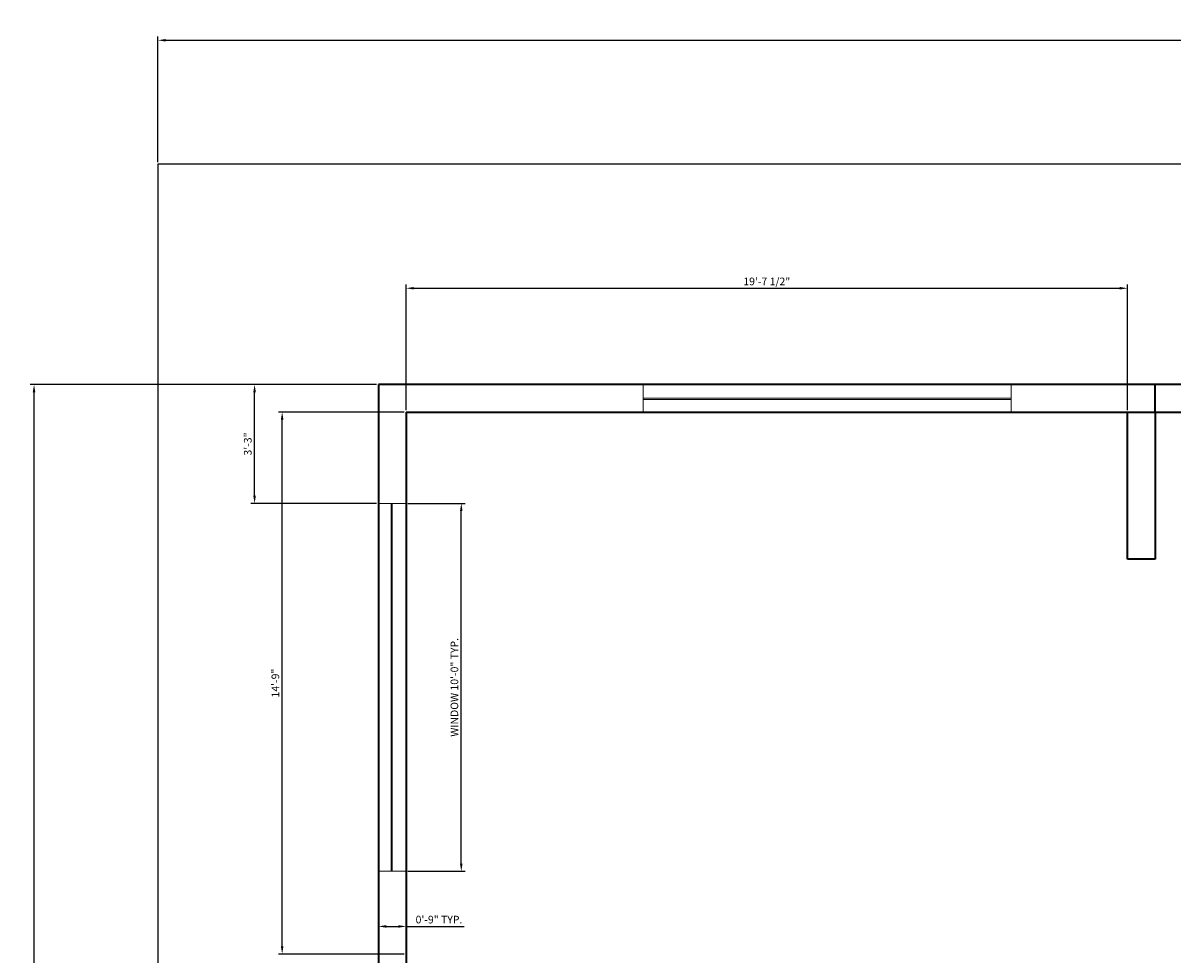
# Model space of a CAD drawing. Units: inches. Extents: x 250205121 to 250208111, y 89832590 to 89833271.
# Tile 12 of 14: x 250207223 to 250207599, y 89832955 to 89833259. Entities that reach past the tile are written whole.
import ezdxf

# ---------------------------------------------------------------- set-up
doc = ezdxf.new("R2010")
doc.units = ezdxf.units.IN
for name, color, linetype, lineweight in [('A-WALL', 7, 'Continuous', 35), ('C-PROP', 8, 'Continuous', 25), ('dimensions', 2, 'Continuous', 18), ('window', 4, 'Continuous', 18)]:
    doc.layers.add(name, color=color, linetype=linetype, lineweight=lineweight)
doc.styles.get("Standard").update_dxf_attribs({"font": 'arial.ttf'})
doc.dimstyles.new('ISO-25', dxfattribs={"dimtxt": 2.5, "dimasz": 2.5, "dimexe": 1.25, "dimexo": 0.625, "dimtad": 1, "dimlunit": 4, "dimtxsty": 'Standard', "dimcen": 2.5, "dimadec": 0, "dimazin": 0, "dimtfac": 1, "dimtmove": 0, "dimatfit": 3, "dimfxl": 1, "dimarcsym": 0})

# ---------------------------------------------------------------- blocks, each defined once
blk = doc.blocks.new('WIN-120IN')
for p, q in [((0, 19), (0, 120.13)), ((0, 120.13), (9, 120.13)), ((4.1, 0), (4.1, 120.13)), ((4.5, 0), (4.5, 120.13)), ((9, 120.13), (9, 0)), ((0, 19), (0, 0)), ((9, 0), (0, 0))]:
    blk.add_line(p, q)
blk = doc.blocks.new('*D35')
at = {"layer": 'Defpoints', "color": 0, "transparency": 16777216}
for p in [(250207348.21, 89833102.38), (250207366.23, 89833102.38), (250207348.21, 89832982.25)]:
    blk.add_point(p, dxfattribs=at)
at = {"layer": 'dimensions', "color": 0, "lineweight": -2, "transparency": 16777216}
for p, q in [((250207348.83, 89833102.38), (250207367.48, 89833102.38)), ((250207366.23, 89832984.75), (250207366.23, 89833099.88)), ((250207348.83, 89832982.25), (250207367.48, 89832982.25))]:
    blk.add_line(p, q, dxfattribs=at)
at = {"layer": 'dimensions', "color": 0, "transparency": 16777216}
for points in [[(250207365.81, 89833099.88), (250207366.64, 89833099.88), (250207366.23, 89833102.38)], [(250207365.81, 89832984.75), (250207366.64, 89832984.75), (250207366.23, 89832982.25)]]:
    blk.add_solid(points, dxfattribs=at)
at = {"layer": 'dimensions', "color": 0, "transparency": 16777216, "insert": (250207364.31, 89833042.31), "char_height": 2.5, "attachment_point": 5, "rotation": 90}
blk.add_mtext('WINDOW 10\'-0" TYP.', dxfattribs=at)
blk = doc.blocks.new('*D36')
at = {"layer": 'Defpoints', "color": 0, "transparency": 16777216}
for p in [(250207339.21, 89832982.25), (250207348.21, 89832982.25), (250207348.21, 89832964.23)]:
    blk.add_point(p, dxfattribs=at)
at = {"layer": 'dimensions', "color": 0, "lineweight": -2, "transparency": 16777216}
for p, q in [((250207339.21, 89832981.62), (250207339.21, 89832962.98)), ((250207348.21, 89832981.62), (250207348.21, 89832962.98)), ((250207341.71, 89832964.23), (250207345.71, 89832964.23)), ((250207348.21, 89832964.23), (250207367.2, 89832964.23))]:
    blk.add_line(p, q, dxfattribs=at)
at = {"layer": 'dimensions', "color": 0, "transparency": 16777216}
for points in [[(250207341.71, 89832964.64), (250207341.71, 89832963.81), (250207339.21, 89832964.23)], [(250207345.71, 89832964.64), (250207345.71, 89832963.81), (250207348.21, 89832964.23)]]:
    blk.add_solid(points, dxfattribs=at)
at = {"layer": 'dimensions', "color": 0, "transparency": 16777216, "insert": (250207358.95, 89832966.13), "char_height": 2.5, "attachment_point": 5}
blk.add_mtext('0\'-9" TYP.', dxfattribs=at)
blk = doc.blocks.new('*D66')
at = {"layer": 'Defpoints', "color": 0, "transparency": 16777216}
for p in [(250208069.71, 89833253.67), (250207267.21, 89833213.22), (250208069.71, 89833213.22)]:
    blk.add_point(p, dxfattribs=at)
at = {"layer": 'dimensions', "color": 0, "lineweight": -2, "transparency": 16777216}
for p, q in [((250207267.21, 89833213.84), (250207267.21, 89833254.92)), ((250208069.71, 89833213.84), (250208069.71, 89833254.92)), ((250207269.71, 89833253.67), (250208067.21, 89833253.67))]:
    blk.add_line(p, q, dxfattribs=at)
at = {"layer": 'dimensions', "color": 0, "transparency": 16777216}
for points in [[(250207269.71, 89833254.08), (250207269.71, 89833253.25), (250207267.21, 89833253.67)], [(250208067.21, 89833254.08), (250208067.21, 89833253.25), (250208069.71, 89833253.67)]]:
    blk.add_solid(points, dxfattribs=at)
at = {"layer": 'dimensions', "color": 0, "transparency": 16777216, "insert": (250207668.46, 89833255.58), "char_height": 2.5, "attachment_point": 5}
blk.add_mtext('66\'-10 1/2"', dxfattribs=at)
blk = doc.blocks.new('*D71')
at = {"layer": 'Defpoints', "color": 0, "transparency": 16777216}
for p in [(250207226.76, 89833141.22), (250207339.21, 89833141.22), (250207339.21, 89832712.22)]:
    blk.add_point(p, dxfattribs=at)
at = {"layer": 'dimensions', "color": 0, "lineweight": -2, "transparency": 16777216}
for p, q in [((250207338.58, 89833141.22), (250207225.51, 89833141.22)), ((250207226.76, 89832714.72), (250207226.76, 89833138.72)), ((250207338.58, 89832712.22), (250207225.51, 89832712.22))]:
    blk.add_line(p, q, dxfattribs=at)
at = {"layer": 'dimensions', "color": 0, "transparency": 16777216}
for points in [[(250207226.34, 89833138.72), (250207227.17, 89833138.72), (250207226.76, 89833141.22)], [(250207226.34, 89832714.72), (250207227.17, 89832714.72), (250207226.76, 89832712.22)]]:
    blk.add_solid(points, dxfattribs=at)
at = {"layer": 'dimensions', "color": 0, "transparency": 16777216, "insert": (250207224.85, 89832926.72), "char_height": 2.5, "attachment_point": 5, "rotation": 90}
blk.add_mtext('35\'-9"', dxfattribs=at)
blk = doc.blocks.new('*D73')
at = {"layer": 'Defpoints', "color": 0, "transparency": 16777216}
for p in [(250207583.71, 89833172.67), (250207348.21, 89833132.22), (250207583.71, 89833132.22)]:
    blk.add_point(p, dxfattribs=at)
at = {"layer": 'dimensions', "color": 0, "lineweight": -2, "transparency": 16777216}
for p, q in [((250207348.21, 89833132.84), (250207348.21, 89833173.92)), ((250207350.71, 89833172.67), (250207581.21, 89833172.67)), ((250207583.71, 89833132.84), (250207583.71, 89833173.92))]:
    blk.add_line(p, q, dxfattribs=at)
at = {"layer": 'dimensions', "color": 0, "transparency": 16777216}
for points in [[(250207350.71, 89833173.08), (250207350.71, 89833172.25), (250207348.21, 89833172.67)], [(250207581.21, 89833173.08), (250207581.21, 89833172.25), (250207583.71, 89833172.67)]]:
    blk.add_solid(points, dxfattribs=at)
at = {"layer": 'dimensions', "color": 0, "transparency": 16777216, "insert": (250207465.96, 89833174.58), "char_height": 2.5, "attachment_point": 5}
blk.add_mtext('19\'-7 1/2"', dxfattribs=at)
blk = doc.blocks.new('*D74')
at = {"layer": 'Defpoints', "color": 0, "transparency": 16777216}
for p in [(250207307.76, 89833132.22), (250207348.21, 89833132.22), (250207348.21, 89832955.22)]:
    blk.add_point(p, dxfattribs=at)
at = {"layer": 'dimensions', "color": 0, "lineweight": -2, "transparency": 16777216}
for p, q in [((250207347.58, 89833132.22), (250207306.51, 89833132.22)), ((250207307.76, 89832957.72), (250207307.76, 89833129.72)), ((250207347.58, 89832955.22), (250207306.51, 89832955.22))]:
    blk.add_line(p, q, dxfattribs=at)
at = {"layer": 'dimensions', "color": 0, "transparency": 16777216}
for points in [[(250207307.34, 89833129.72), (250207308.17, 89833129.72), (250207307.76, 89833132.22)], [(250207307.34, 89832957.72), (250207308.17, 89832957.72), (250207307.76, 89832955.22)]]:
    blk.add_solid(points, dxfattribs=at)
at = {"layer": 'dimensions', "color": 0, "transparency": 16777216, "insert": (250207305.86, 89833043.72), "char_height": 2.5, "attachment_point": 5, "rotation": 90}
blk.add_mtext('14\'-9"', dxfattribs=at)
blk = doc.blocks.new('*D75')
at = {"layer": 'Defpoints', "color": 0, "transparency": 16777216}
for p in [(250207298.76, 89833141.22), (250207339.21, 89833141.22), (250207339.21, 89833102.38)]:
    blk.add_point(p, dxfattribs=at)
at = {"layer": 'dimensions', "color": 0, "lineweight": -2, "transparency": 16777216}
for p, q in [((250207338.58, 89833141.22), (250207297.51, 89833141.22)), ((250207298.76, 89833104.88), (250207298.76, 89833138.72)), ((250207338.58, 89833102.38), (250207297.51, 89833102.38))]:
    blk.add_line(p, q, dxfattribs=at)
at = {"layer": 'dimensions', "color": 0, "transparency": 16777216}
for points in [[(250207298.34, 89833138.72), (250207299.17, 89833138.72), (250207298.76, 89833141.22)], [(250207298.34, 89833104.88), (250207299.17, 89833104.88), (250207298.76, 89833102.38)]]:
    blk.add_solid(points, dxfattribs=at)
at = {"layer": 'dimensions', "color": 0, "transparency": 16777216, "insert": (250207296.85, 89833121.8), "char_height": 2.5, "attachment_point": 5, "rotation": 90}
blk.add_mtext('3\'-3"', dxfattribs=at)

msp = doc.modelspace()

# ---------------------------------------------------------------- linework, layer by layer
at = {"layer": 'A-WALL'}
for p, q in [((250207348.207, 89833141.217), (250207339.207, 89833141.217)), ((250207339.207, 89833141.217), (250207339.207, 89833132.217)), ((250207970.867, 89833141.217), (250207348.207, 89833141.217)), ((250207592.707, 89833132.217), (250207592.707, 89833141.217)), ((250207339.207, 89833132.217), (250207339.207, 89833089.717)), ((250207348.207, 89833132.217), (250207966.367, 89833132.217)), ((250207348.207, 89833132.217), (250207348.207, 89833089.717)), ((250207583.707, 89833084.217), (250207583.707, 89833132.217)), ((250207592.707, 89833132.217), (250207592.707, 89833084.217)), ((250207339.207, 89833089.717), (250207339.207, 89832712.217)), ((250207348.207, 89833089.717), (250207348.207, 89832721.217)), ((250207592.707, 89833084.217), (250207583.707, 89833084.217))]:
    msp.add_line(p, q, dxfattribs=at)
at = {"layer": 'C-PROP'}
for p, q in [((250207592.707, 89833213.217), (250207267.207, 89833213.217)), ((250207267.207, 89833213.217), (250207267.207, 89832640.217)), ((250208069.707, 89833213.217), (250207592.707, 89833213.217))]:
    msp.add_line(p, q, dxfattribs=at)

# ---------------------------------------------------------------- block references
at = {"layer": 'window', "rotation": 90.000000015914}
msp.add_blockref('WIN-120IN', (250207545.693, 89833132.217), dxfattribs=at)
at = {"layer": 'window'}
msp.add_blockref('WIN-120IN', (250207339.207, 89832982.248), dxfattribs=at)

# ---------------------------------------------------------------- dimensions: what is measured, and where the dimension line sits
at = {"layer": 'dimensions'}
for base, p1, p2, picture, middle in [((250208069.707, 89833253.667), (250207267.207, 89833213.217), (250208069.707, 89833213.217), '*D66', (250207668.457, 89833255.585)), ((250207583.707, 89833172.667), (250207348.207, 89833132.217), (250207583.707, 89833132.217), '*D73', (250207465.957, 89833174.585))]:
    dim = msp.add_linear_dim(base=base, p1=p1, p2=p2, dimstyle='ISO-25', override={"dimdec": 1, "dimlfac": 1, "dimrnd": 0, "dimzin": 1, "dimdsep": 46, "dimlunit": 4, "dimfrac": 2}, dxfattribs=at)
    dim.commit()
    dim.dimension.update_dxf_attribs({"geometry": picture, "text_midpoint": middle})
for base, p1, p2, picture, middle in [((250207226.757, 89833141.217), (250207339.207, 89832712.217), (250207339.207, 89833141.217), '*D71', (250207224.855, 89832926.717)), ((250207298.757, 89833141.217), (250207339.207, 89833102.38), (250207339.207, 89833141.217), '*D75', (250207296.855, 89833121.799)), ((250207307.757, 89833132.217), (250207348.207, 89832955.217), (250207348.207, 89833132.217), '*D74', (250207305.856, 89833043.717))]:
    dim = msp.add_linear_dim(base=base, p1=p1, p2=p2, angle=90, dimstyle='ISO-25', override={"dimdec": 1, "dimlfac": 1, "dimrnd": 0, "dimzin": 1, "dimdsep": 46, "dimlunit": 4, "dimfrac": 2}, dxfattribs=at)
    dim.commit()
    dim.dimension.update_dxf_attribs({"geometry": picture, "text_midpoint": middle})
dim = msp.add_linear_dim(base=(250207366.227, 89833102.38), p1=(250207348.207, 89832982.248), p2=(250207348.207, 89833102.38), angle=90, text='WINDOW <> TYP.', dimstyle='ISO-25', override={"dimdec": 1, "dimlfac": 1, "dimrnd": 0, "dimzin": 1, "dimdsep": 46, "dimlunit": 4, "dimfrac": 2}, dxfattribs=at)
dim.commit()
dim.dimension.update_dxf_attribs({"geometry": '*D35', "text_midpoint": (250207364.308, 89833042.314)})
dim = msp.add_linear_dim(base=(250207348.207, 89832964.228), p1=(250207339.207, 89832982.248), p2=(250207348.207, 89832982.248), text='<> TYP.', dimstyle='ISO-25', override={"dimdec": 1, "dimlfac": 1, "dimrnd": 0, "dimzin": 1, "dimdsep": 46, "dimlunit": 4, "dimfrac": 2}, dxfattribs=at)
dim.commit()
dim.dimension.update_dxf_attribs({"geometry": '*D36', "text_midpoint": (250207358.951, 89832966.13)})

doc.saveas('drawing.dxf')
